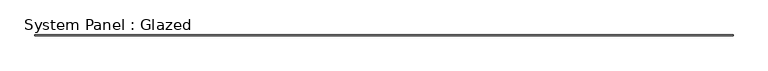
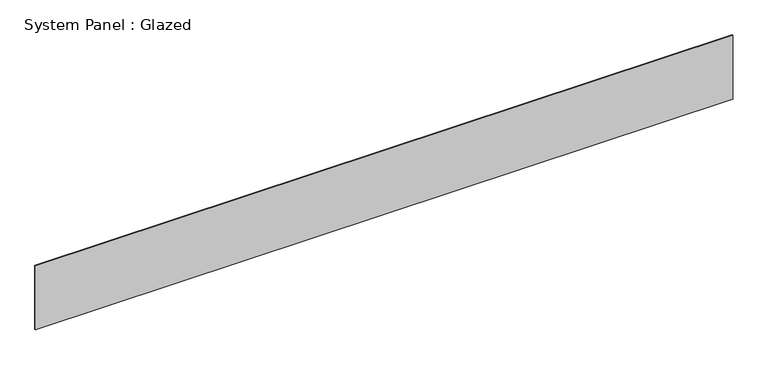
"""IFC4 building model written with IfcOpenShell, lengths in millimetres: plate geometry, System Panel : Glazed."""

from ifc_helpers import new_model, si_unit, origin, origin_with_axes, place, context, project, spatial, polyline, outline, extrude, source, transform, mapped, element, save


def system_panel_glazed_f8a0c966(model_context):
    return source(origin(), model_context, "Body", "SweptSolid", [
        extrude(outline(polyline([(11049.0, 19.05), (-11049.0, 19.05), (-11049.0, 44.45), (11049.0, 44.45), (11049.0, 19.05)])), origin_with_axes(), (0.0, 0.0, 1.0), 2141.8122839),
    ])


if __name__ == "__main__":
    model = new_model("IFC4")
    model_context = context("Model", 3, world=origin())
    ifc_project = project(units=[si_unit("LENGTHUNIT", "METRE", prefix="MILLI")], contexts=[model_context])
    site = spatial("IfcSite", under=ifc_project)
    building = spatial("IfcBuilding", under=site)
    placement = place(None, origin())
    system_panel_glazed_shape = system_panel_glazed_f8a0c966(model_context)
    element("IfcPlate", 1, ObjectType="System Panel : Glazed", at=placement, inside=building, context=model_context, shape_type="MappedRepresentation", body=[
        mapped(system_panel_glazed_shape, transform((0.0, 0.0, 0.0), x_axis=(1.0, 0.0, 0.0), y_axis=(0.0, 1.0, 0.0), z_axis=(0.0, 0.0, 1.0))),
    ])
    save(model, "model.ifc")

# Revit data of these elements
# Type "System Panel : Glazed"
#   Construction Type Id = "GSP4R"
#   Analytic Construction = "1/8 in Pilkington single glazing"
#   Visual Light Transmittance = 0.9
#   Solar Heat Gain Coefficient = 0.86
#   Heat Transfer Coefficient (U) = 1.18115 BTU/(h·ft²·°F)
# Element 1 (IfcPlate, "System Panel : Glazed")
#   Materials on its faces: "Glass"
# Materials
#   "Glass": class "Glass", colour RGB 0 128 192, transparency 0.75, Description = "Soda Lime Glass", Cost = 0
